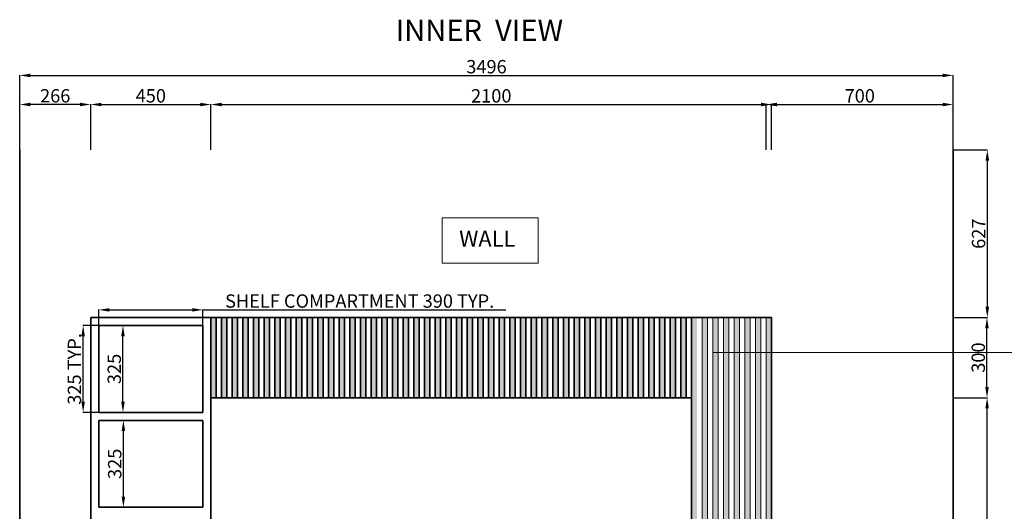
# Model space of a CAD drawing. Units: millimetres. Extents: x 11439 to 24661, y -4767 to -6.
# Tile 4 of 5: x 18965 to 22652, y -2690 to -851. Entities that reach past the tile are written whole.
import ezdxf

# ---------------------------------------------------------------- set-up
doc = ezdxf.new("R2010")
doc.units = ezdxf.units.MM
for name, color, linetype, lineweight in [('A-ANNO-DIMS', 2, 'Continuous', 18), ('A-ANNO-TEXT', 3, 'Continuous', 18), ('A-FURN', 7, 'Continuous', 35), ('A-FURN-PATT', 8, 'Continuous', 13)]:
    doc.layers.add(name, color=color, linetype=linetype, lineweight=lineweight)
doc.styles.get("Standard").update_dxf_attribs({"font": 'arial.ttf'})
doc.dimstyles.new('ISO-25', dxfattribs={"dimtxt": 50, "dimasz": 40, "dimexe": 1.25, "dimexo": 0.625, "dimtad": 1, "dimtxsty": 'Standard', "dimcen": 2.5, "dimadec": 0, "dimazin": 0, "dimtfac": 1, "dimtmove": 0, "dimatfit": 3, "dimfxl": 1, "dimarcsym": 0})

# ---------------------------------------------------------------- blocks, each defined once
blk = doc.blocks.new('*D28')
at = {"layer": 'A-ANNO-DIMS', "color": 0, "lineweight": -2, "transparency": 16777216}
for p, q in [((22461.4, -2264.7), (22588.9, -2264.7)), ((22587.6, -3424.7), (22587.6, -2304.7)), ((22461.4, -3464.7), (22588.9, -3464.7))]:
    blk.add_line(p, q, dxfattribs=at)
at = {"layer": 'A-ANNO-DIMS', "color": 0, "transparency": 16777216}
for points in [[(22581, -2304.7), (22594.3, -2304.7), (22587.6, -2264.7)], [(22581, -3424.7), (22594.3, -3424.7), (22587.6, -3464.7)]]:
    blk.add_solid(points, dxfattribs=at)
at = {"layer": 'Defpoints', "color": 0, "transparency": 16777216}
for p in [(22460.8, -2264.7), (22587.6, -2264.7), (22460.8, -3464.7)]:
    blk.add_point(p, dxfattribs=at)
at = {"layer": 'A-ANNO-DIMS', "color": 0, "transparency": 16777216, "insert": (22561.5, -2864.7), "char_height": 50, "attachment_point": 5, "rotation": 90}
blk.add_mtext('1200', dxfattribs=at)
blk = doc.blocks.new('*D29')
at = {"layer": 'A-ANNO-DIMS', "color": 0, "lineweight": -2, "transparency": 16777216}
for p, q in [((22465.2, -1964.7), (22588.5, -1964.7)), ((22587.2, -2224.7), (22587.2, -2004.7)), ((22461.4, -2264.7), (22588.5, -2264.7))]:
    blk.add_line(p, q, dxfattribs=at)
at = {"layer": 'A-ANNO-DIMS', "color": 0, "transparency": 16777216}
for points in [[(22580.5, -2004.7), (22593.9, -2004.7), (22587.2, -1964.7)], [(22580.5, -2224.7), (22593.9, -2224.7), (22587.2, -2264.7)]]:
    blk.add_solid(points, dxfattribs=at)
at = {"layer": 'Defpoints', "color": 0, "transparency": 16777216}
for p in [(22464.5, -1964.7), (22587.2, -1964.7), (22460.8, -2264.7)]:
    blk.add_point(p, dxfattribs=at)
at = {"layer": 'A-ANNO-DIMS', "color": 0, "transparency": 16777216, "insert": (22561, -2114.7), "char_height": 50, "attachment_point": 5, "rotation": 90}
blk.add_mtext('300', dxfattribs=at)
blk = doc.blocks.new('*D23')
at = {"layer": 'A-ANNO-DIMS', "color": 0, "lineweight": -2, "transparency": 16777216}
for p, q in [((18964.8, -1337.1), (18964.8, -1166.8)), ((19190.8, -1168), (19004.8, -1168)), ((19230.8, -1337.1), (19230.8, -1166.8))]:
    blk.add_line(p, q, dxfattribs=at)
at = {"layer": 'A-ANNO-DIMS', "color": 0, "transparency": 16777216}
for points in [[(19004.8, -1161.4), (19004.8, -1174.7), (18964.8, -1168)], [(19190.8, -1161.4), (19190.8, -1174.7), (19230.8, -1168)]]:
    blk.add_solid(points, dxfattribs=at)
at = {"layer": 'Defpoints', "color": 0, "transparency": 16777216}
for p in [(18964.8, -1168), (18964.8, -1337.7), (19230.8, -1337.7)]:
    blk.add_point(p, dxfattribs=at)
at = {"layer": 'A-ANNO-DIMS', "color": 0, "transparency": 16777216, "insert": (19097.8, -1141.9), "char_height": 50, "attachment_point": 5}
blk.add_mtext('266', dxfattribs=at)
blk = doc.blocks.new('*D24')
at = {"layer": 'A-ANNO-DIMS', "color": 0, "lineweight": -2, "transparency": 16777216}
for p, q in [((19230.8, -1337.1), (19230.8, -1166.8)), ((19270.8, -1168), (19640.8, -1168)), ((19680.8, -1337.1), (19680.8, -1166.8))]:
    blk.add_line(p, q, dxfattribs=at)
at = {"layer": 'A-ANNO-DIMS', "color": 0, "transparency": 16777216}
for points in [[(19270.8, -1161.4), (19270.8, -1174.7), (19230.8, -1168)], [(19640.8, -1161.4), (19640.8, -1174.7), (19680.8, -1168)]]:
    blk.add_solid(points, dxfattribs=at)
at = {"layer": 'Defpoints', "color": 0, "transparency": 16777216}
for p in [(19680.8, -1168), (19230.8, -1337.7), (19680.8, -1337.7)]:
    blk.add_point(p, dxfattribs=at)
at = {"layer": 'A-ANNO-DIMS', "color": 0, "transparency": 16777216, "insert": (19455.8, -1141.9), "char_height": 50, "attachment_point": 5}
blk.add_mtext('450', dxfattribs=at)
blk = doc.blocks.new('*D25')
at = {"layer": 'A-ANNO-DIMS', "color": 0, "lineweight": -2, "transparency": 16777216}
for p, q in [((19680.8, -1337.1), (19680.8, -1166.9)), ((19720.8, -1168.1), (21740.8, -1168.1)), ((21780.8, -1337.1), (21780.8, -1166.9))]:
    blk.add_line(p, q, dxfattribs=at)
at = {"layer": 'A-ANNO-DIMS', "color": 0, "transparency": 16777216}
for points in [[(19720.8, -1161.4), (19720.8, -1174.8), (19680.8, -1168.1)], [(21740.8, -1161.4), (21740.8, -1174.8), (21780.8, -1168.1)]]:
    blk.add_solid(points, dxfattribs=at)
at = {"layer": 'Defpoints', "color": 0, "transparency": 16777216}
for p in [(21780.8, -1168.1), (19680.8, -1337.7), (21780.8, -1337.7)]:
    blk.add_point(p, dxfattribs=at)
at = {"layer": 'A-ANNO-DIMS', "color": 0, "transparency": 16777216, "insert": (20730.8, -1142), "char_height": 50, "attachment_point": 5}
blk.add_mtext('2100', dxfattribs=at)
blk = doc.blocks.new('*D36')
at = {"layer": 'A-ANNO-DIMS', "color": 0, "lineweight": -2, "transparency": 16777216}
for p, q in [((21760.8, -1337.1), (21760.8, -1166.9)), ((21800.8, -1168.1), (22420.8, -1168.1)), ((22460.8, -1337.1), (22460.8, -1166.9))]:
    blk.add_line(p, q, dxfattribs=at)
at = {"layer": 'A-ANNO-DIMS', "color": 0, "transparency": 16777216}
for points in [[(21800.8, -1161.4), (21800.8, -1174.8), (21760.8, -1168.1)], [(22420.8, -1161.4), (22420.8, -1174.8), (22460.8, -1168.1)]]:
    blk.add_solid(points, dxfattribs=at)
at = {"layer": 'Defpoints', "color": 0, "transparency": 16777216}
for p in [(22460.8, -1168.1), (21760.8, -1337.7), (22460.8, -1337.7)]:
    blk.add_point(p, dxfattribs=at)
at = {"layer": 'A-ANNO-DIMS', "color": 0, "transparency": 16777216, "insert": (22110.8, -1142), "char_height": 50, "attachment_point": 5}
blk.add_mtext('700', dxfattribs=at)
blk = doc.blocks.new('*D30')
at = {"layer": 'A-ANNO-DIMS', "color": 0, "lineweight": -2, "transparency": 16777216}
for p, q in [((22461.4, -1337.7), (22589.7, -1337.7)), ((22588.5, -1377.7), (22588.5, -1924.7)), ((22465.2, -1964.7), (22589.7, -1964.7))]:
    blk.add_line(p, q, dxfattribs=at)
at = {"layer": 'A-ANNO-DIMS', "color": 0, "transparency": 16777216}
for points in [[(22581.8, -1377.7), (22595.1, -1377.7), (22588.5, -1337.7)], [(22581.8, -1924.7), (22595.1, -1924.7), (22588.5, -1964.7)]]:
    blk.add_solid(points, dxfattribs=at)
at = {"layer": 'Defpoints', "color": 0, "transparency": 16777216}
for p in [(22460.8, -1337.7), (22464.5, -1964.7), (22588.5, -1964.7)]:
    blk.add_point(p, dxfattribs=at)
at = {"layer": 'A-ANNO-DIMS', "color": 0, "transparency": 16777216, "insert": (22562.3, -1651.2), "char_height": 50, "attachment_point": 5, "rotation": 90}
blk.add_mtext('627', dxfattribs=at)
blk = doc.blocks.new('*D41')
at = {"layer": 'A-ANNO-DIMS', "color": 0, "lineweight": -2, "transparency": 16777216}
for p, q in [((19261.4, -2349.7), (19354.4, -2349.7)), ((19353.1, -2634.7), (19353.1, -2389.7)), ((19261.4, -2674.7), (19354.4, -2674.7))]:
    blk.add_line(p, q, dxfattribs=at)
at = {"layer": 'A-ANNO-DIMS', "color": 0, "transparency": 16777216}
for points in [[(19346.5, -2389.7), (19359.8, -2389.7), (19353.1, -2349.7)], [(19346.5, -2634.7), (19359.8, -2634.7), (19353.1, -2674.7)]]:
    blk.add_solid(points, dxfattribs=at)
at = {"layer": 'Defpoints', "color": 0, "transparency": 16777216}
for p in [(19260.8, -2349.7), (19353.1, -2349.7), (19260.8, -2674.7)]:
    blk.add_point(p, dxfattribs=at)
at = {"layer": 'A-ANNO-DIMS', "color": 0, "transparency": 16777216, "insert": (19327, -2512.2), "char_height": 50, "attachment_point": 5, "rotation": 90}
blk.add_mtext('325', dxfattribs=at)
blk = doc.blocks.new('*D42')
at = {"layer": 'A-ANNO-DIMS', "color": 0, "lineweight": -2, "transparency": 16777216}
for p, q in [((19261.4, -1994.7), (19352.7, -1994.7)), ((19351.5, -2279.7), (19351.5, -2034.7)), ((19261.4, -2319.7), (19352.7, -2319.7))]:
    blk.add_line(p, q, dxfattribs=at)
at = {"layer": 'A-ANNO-DIMS', "color": 0, "transparency": 16777216}
for points in [[(19344.8, -2034.7), (19358.2, -2034.7), (19351.5, -1994.7)], [(19344.8, -2279.7), (19358.2, -2279.7), (19351.5, -2319.7)]]:
    blk.add_solid(points, dxfattribs=at)
at = {"layer": 'Defpoints', "color": 0, "transparency": 16777216}
for p in [(19260.8, -1994.7), (19351.5, -1994.7), (19260.8, -2319.7)]:
    blk.add_point(p, dxfattribs=at)
at = {"layer": 'A-ANNO-DIMS', "color": 0, "transparency": 16777216, "insert": (19325.3, -2157.2), "char_height": 50, "attachment_point": 5, "rotation": 90}
blk.add_mtext('325', dxfattribs=at)
blk = doc.blocks.new('SHELF-COMPARTMENT')
for p, q in [((0, 325), (390, 325)), ((0, 0), (0, 325)), ((390, 0), (390, 325)), ((0, 0), (390, 0))]:
    blk.add_line(p, q)
blk = doc.blocks.new('*D47')
at = {"layer": 'A-ANNO-DIMS', "color": 0, "lineweight": -2, "transparency": 16777216}
for p, q in [((19260.8, -1994.1), (19260.8, -1934.9)), ((19300.8, -1936.2), (19610.8, -1936.2)), ((19650.8, -1994.1), (19650.8, -1934.9)), ((19650.8, -1936.2), (20785.1, -1936.2))]:
    blk.add_line(p, q, dxfattribs=at)
at = {"layer": 'A-ANNO-DIMS', "color": 0, "transparency": 16777216}
for points in [[(19300.8, -1929.5), (19300.8, -1942.9), (19260.8, -1936.2)], [(19610.8, -1929.5), (19610.8, -1942.9), (19650.8, -1936.2)]]:
    blk.add_solid(points, dxfattribs=at)
at = {"layer": 'Defpoints', "color": 0, "transparency": 16777216}
for p in [(19650.8, -1936.2), (19260.8, -1994.7), (19650.8, -1994.7)]:
    blk.add_point(p, dxfattribs=at)
at = {"layer": 'A-ANNO-DIMS', "color": 0, "transparency": 16777216, "insert": (20237.9, -1909.7), "char_height": 50, "attachment_point": 5}
blk.add_mtext('SHELF COMPARTMENT 390 TYP.', dxfattribs=at)
blk = doc.blocks.new('*D48')
at = {"layer": 'A-ANNO-DIMS', "color": 0, "lineweight": -2, "transparency": 16777216}
for p, q in [((19260.1, -1994.7), (19201, -1994.7)), ((19202.3, -2279.7), (19202.3, -2034.7)), ((19260.1, -2319.7), (19201, -2319.7))]:
    blk.add_line(p, q, dxfattribs=at)
at = {"layer": 'A-ANNO-DIMS', "color": 0, "transparency": 16777216}
for points in [[(19195.6, -2034.7), (19208.9, -2034.7), (19202.3, -1994.7)], [(19195.6, -2279.7), (19208.9, -2279.7), (19202.3, -2319.7)]]:
    blk.add_solid(points, dxfattribs=at)
at = {"layer": 'Defpoints', "color": 0, "transparency": 16777216}
for p in [(19202.3, -1994.7), (19260.8, -1994.7), (19260.8, -2319.7)]:
    blk.add_point(p, dxfattribs=at)
at = {"layer": 'A-ANNO-DIMS', "color": 0, "transparency": 16777216, "insert": (19176.1, -2157.2), "char_height": 50, "attachment_point": 5, "rotation": 90}
blk.add_mtext('325 TYP.', dxfattribs=at)
blk = doc.blocks.new('*D60')
at = {"layer": 'A-ANNO-DIMS', "color": 0, "lineweight": -2, "transparency": 16777216}
for p, q in [((18964.8, -1337.1), (18964.8, -1057.9)), ((19004.8, -1059.2), (22420.8, -1059.2)), ((22460.8, -1337.1), (22460.8, -1057.9))]:
    blk.add_line(p, q, dxfattribs=at)
at = {"layer": 'A-ANNO-DIMS', "color": 0, "transparency": 16777216}
for points in [[(19004.8, -1052.5), (19004.8, -1065.9), (18964.8, -1059.2)], [(22420.8, -1052.5), (22420.8, -1065.9), (22460.8, -1059.2)]]:
    blk.add_solid(points, dxfattribs=at)
at = {"layer": 'Defpoints', "color": 0, "transparency": 16777216}
for p in [(22460.8, -1059.2), (18964.8, -1337.7), (22460.8, -1337.7)]:
    blk.add_point(p, dxfattribs=at)
at = {"layer": 'A-ANNO-DIMS', "color": 0, "transparency": 16777216, "insert": (20712.8, -1033), "char_height": 50, "attachment_point": 5}
blk.add_mtext('3496', dxfattribs=at)

msp = doc.modelspace()

# ---------------------------------------------------------------- hatches: boundary and pattern name
at = {"layer": 'A-FURN-PATT'}
h = msp.add_hatch(color=256, dxfattribs=at)
h.dxf.hatch_style = 1
h.paths.add_polyline_path([(19700.761, -3464.684), (19680.761, -3464.684), (19680.761, -3764.684), (19700.761, -3764.684)])
h.paths.add_polyline_path([(19740.761, -3464.684), (19720.761, -3464.684), (19720.761, -3764.684), (19740.761, -3764.684)])
h.paths.add_polyline_path([(19780.761, -3464.684), (19760.761, -3464.684), (19760.761, -3764.684), (19780.761, -3764.684)])
h.paths.add_polyline_path([(19800.761, -3764.684), (19820.761, -3764.684), (19820.761, -3464.684), (19800.761, -3464.684)])
h.paths.add_polyline_path([(19860.761, -3464.684), (19840.761, -3464.684), (19840.761, -3764.684), (19860.761, -3764.684)])
h.paths.add_polyline_path([(19900.761, -3464.684), (19880.761, -3464.684), (19880.761, -3764.684), (19900.761, -3764.684)])
h.paths.add_polyline_path([(19940.761, -3464.684), (19920.761, -3464.684), (19920.761, -3764.684), (19940.761, -3764.684)])
h.paths.add_polyline_path([(19960.761, -3764.684), (19980.761, -3764.684), (19980.761, -3464.684), (19960.761, -3464.684)])
h.paths.add_polyline_path([(20020.761, -3464.684), (20000.761, -3464.684), (20000.761, -3764.684), (20020.761, -3764.684)])
h.paths.add_polyline_path([(20040.761, -3764.684), (20060.761, -3764.684), (20060.761, -3464.684), (20040.761, -3464.684)])
h.paths.add_polyline_path([(20080.761, -3764.684), (20100.761, -3764.684), (20100.761, -3464.684), (20080.761, -3464.684)])
h.paths.add_polyline_path([(20140.761, -3464.684), (20120.761, -3464.684), (20120.761, -3764.684), (20140.761, -3764.684)])
h.paths.add_polyline_path([(20160.761, -3764.684), (20180.761, -3764.684), (20180.761, -3464.684), (20160.761, -3464.684)])
h.paths.add_polyline_path([(20220.761, -3464.684), (20200.761, -3464.684), (20200.761, -3764.684), (20220.761, -3764.684)])
h.paths.add_polyline_path([(20240.761, -3764.684), (20260.761, -3764.684), (20260.761, -3464.684), (20240.761, -3464.684)])
h.paths.add_polyline_path([(20300.761, -3464.684), (20280.761, -3464.684), (20280.761, -3764.684), (20300.761, -3764.684)])
h.paths.add_polyline_path([(20340.761, -3464.684), (20320.761, -3464.684), (20320.761, -3764.684), (20340.761, -3764.684)])
h.paths.add_polyline_path([(20360.761, -3764.684), (20380.761, -3764.684), (20380.761, -3464.684), (20360.761, -3464.684)])
h.paths.add_polyline_path([(20400.761, -3764.684), (20420.761, -3764.684), (20420.761, -3464.684), (20400.761, -3464.684)])
h.paths.add_polyline_path([(20440.761, -3764.684), (20460.761, -3764.684), (20460.761, -3464.684), (20440.761, -3464.684)])
h.paths.add_polyline_path([(20480.761, -3764.684), (20500.761, -3764.684), (20500.761, -3464.684), (20480.761, -3464.684)])
h.paths.add_polyline_path([(20520.761, -3764.684), (20540.761, -3764.684), (20540.761, -3464.684), (20520.761, -3464.684)])
h.paths.add_polyline_path([(20560.761, -3764.684), (20580.761, -3764.684), (20580.761, -3464.684), (20560.761, -3464.684)])
h.paths.add_polyline_path([(20600.761, -3764.684), (20620.761, -3764.684), (20620.761, -3464.684), (20600.761, -3464.684)])
h.paths.add_polyline_path([(20660.761, -3464.684), (20640.761, -3464.684), (20640.761, -3764.684), (20660.761, -3764.684)])
h.paths.add_polyline_path([(20680.761, -3764.684), (20700.761, -3764.684), (20700.761, -3464.684), (20680.761, -3464.684)])
h.paths.add_polyline_path([(20740.761, -3464.684), (20720.761, -3464.684), (20720.761, -3764.684), (20740.761, -3764.684)])
h.paths.add_polyline_path([(20760.761, -3764.684), (20780.761, -3764.684), (20780.761, -3464.684), (20760.761, -3464.684)])
h.paths.add_polyline_path([(20800.761, -3764.684), (20820.761, -3764.684), (20820.761, -3464.684), (20800.761, -3464.684)])
h.paths.add_polyline_path([(20840.761, -3764.684), (20860.761, -3764.684), (20860.761, -3464.684), (20840.761, -3464.684)])
h.paths.add_polyline_path([(20900.761, -3464.684), (20880.761, -3464.684), (20880.761, -3764.684), (20900.761, -3764.684)])
h.paths.add_polyline_path([(20940.761, -3464.684), (20920.761, -3464.684), (20920.761, -3764.684), (20940.761, -3764.684)])
h.paths.add_polyline_path([(20980.761, -3464.684), (20960.761, -3464.684), (20960.761, -3764.684), (20980.761, -3764.684)])
h.paths.add_polyline_path([(21020.761, -3464.684), (21000.761, -3464.684), (21000.761, -3764.684), (21020.761, -3764.684)])
h.paths.add_polyline_path([(21060.761, -3464.684), (21040.761, -3464.684), (21040.761, -3764.684), (21060.761, -3764.684)])
h.paths.add_polyline_path([(21080.761, -3764.684), (21100.761, -3764.684), (21100.761, -3464.684), (21080.761, -3464.684)])
h.paths.add_polyline_path([(21120.761, -3764.684), (21140.761, -3764.684), (21140.761, -3464.684), (21120.761, -3464.684)])
h.paths.add_polyline_path([(21180.761, -3464.684), (21160.761, -3464.684), (21160.761, -3764.684), (21180.761, -3764.684)])
h.paths.add_polyline_path([(21200.761, -3764.684), (21220.761, -3764.684), (21220.761, -3464.684), (21200.761, -3464.684)])
h.paths.add_polyline_path([(21260.761, -3464.684), (21240.761, -3464.684), (21240.761, -3764.684), (21260.761, -3764.684)])
h.paths.add_polyline_path([(21280.761, -3764.684), (21300.761, -3764.684), (21300.761, -3464.684), (21280.761, -3464.684)])
h.paths.add_polyline_path([(21320.761, -3764.684), (21340.761, -3764.684), (21340.761, -3464.684), (21320.761, -3464.684)])
h.paths.add_polyline_path([(21360.761, -3764.684), (21380.761, -3764.684), (21380.761, -3464.684), (21360.761, -3464.684)])
h.paths.add_polyline_path([(21400.761, -3764.684), (21420.761, -3764.684), (21420.761, -3464.684), (21400.761, -3464.684)])
h.paths.add_polyline_path([(21460.761, -3464.684), (21440.761, -3464.684), (21440.761, -3764.684), (21460.761, -3764.684)])
h.paths.add_polyline_path([(19700.761, -1964.684), (19680.761, -1964.684), (19680.761, -2264.684), (19700.761, -2264.684)])
h.paths.add_polyline_path([(19740.761, -1964.684), (19720.761, -1964.684), (19720.761, -2264.684), (19740.761, -2264.684)])
h.paths.add_polyline_path([(19780.761, -1964.684), (19760.761, -1964.684), (19760.761, -2264.684), (19780.761, -2264.684)])
h.paths.add_polyline_path([(19820.761, -1964.684), (19800.761, -1964.684), (19800.761, -2264.684), (19820.761, -2264.684)])
h.paths.add_polyline_path([(19860.761, -2264.684), (19860.761, -1964.684), (19840.761, -1964.684), (19840.761, -2264.684)])
h.paths.add_polyline_path([(19880.761, -2264.684), (19900.761, -2264.684), (19900.761, -1964.684), (19880.761, -1964.684)])
h.paths.add_polyline_path([(19940.761, -1964.684), (19920.761, -1964.684), (19920.761, -2264.684), (19940.761, -2264.684)])
h.paths.add_polyline_path([(19960.761, -2264.684), (19980.761, -2264.684), (19980.761, -1964.684), (19960.761, -1964.684)])
h.paths.add_polyline_path([(20020.761, -1964.684), (20000.761, -1964.684), (20000.761, -2264.684), (20020.761, -2264.684)])
h.paths.add_polyline_path([(20040.761, -2264.684), (20060.761, -2264.684), (20060.761, -1964.684), (20040.761, -1964.684)])
h.paths.add_polyline_path([(20100.761, -1964.684), (20080.761, -1964.684), (20080.761, -2264.684), (20100.761, -2264.684)])
h.paths.add_polyline_path([(20120.761, -2264.684), (20140.761, -2264.684), (20140.761, -1964.684), (20120.761, -1964.684)])
h.paths.add_polyline_path([(20180.761, -1964.684), (20160.761, -1964.684), (20160.761, -2264.684), (20180.761, -2264.684)])
h.paths.add_polyline_path([(20220.761, -1964.684), (20200.761, -1964.684), (20200.761, -2264.684), (20220.761, -2264.684)])
h.paths.add_polyline_path([(20240.761, -2264.684), (20260.761, -2264.684), (20260.761, -1964.684), (20240.761, -1964.684)])
h.paths.add_polyline_path([(20280.761, -2264.684), (20300.761, -2264.684), (20300.761, -1964.684), (20280.761, -1964.684)])
h.paths.add_polyline_path([(20340.761, -1964.684), (20320.761, -1964.684), (20320.761, -2264.684), (20340.761, -2264.684)])
h.paths.add_polyline_path([(20360.761, -2264.684), (20380.761, -2264.684), (20380.761, -1964.684), (20360.761, -1964.684)])
h.paths.add_polyline_path([(20400.761, -2264.684), (20420.761, -2264.684), (20420.761, -1964.684), (20400.761, -1964.684)])
h.paths.add_polyline_path([(20440.761, -2264.684), (20460.761, -2264.684), (20460.761, -1964.684), (20440.761, -1964.684)])
h.paths.add_polyline_path([(20480.761, -2264.684), (20500.761, -2264.684), (20500.761, -1964.684), (20480.761, -1964.684)])
h.paths.add_polyline_path([(20520.761, -2264.684), (20540.761, -2264.684), (20540.761, -1964.684), (20520.761, -1964.684)])
h.paths.add_polyline_path([(20580.761, -1964.684), (20560.761, -1964.684), (20560.761, -2264.684), (20580.761, -2264.684)])
h.paths.add_polyline_path([(20600.761, -2264.684), (20620.761, -2264.684), (20620.761, -1964.684), (20600.761, -1964.684)])
h.paths.add_polyline_path([(20640.761, -2264.684), (20660.761, -2264.684), (20660.761, -1964.684), (20640.761, -1964.684)])
h.paths.add_polyline_path([(20680.761, -2264.684), (20700.761, -2264.684), (20700.761, -1964.684), (20680.761, -1964.684)])
h.paths.add_polyline_path([(20720.761, -2264.684), (20740.761, -2264.684), (20740.761, -1964.684), (20720.761, -1964.684)])
h.paths.add_polyline_path([(20780.761, -1964.684), (20760.761, -1964.684), (20760.761, -2264.684), (20780.761, -2264.684)])
h.paths.add_polyline_path([(20800.761, -2264.684), (20820.761, -2264.684), (20820.761, -1964.684), (20800.761, -1964.684)])
h.paths.add_polyline_path([(20860.761, -1964.684), (20840.761, -1964.684), (20840.761, -2264.684), (20860.761, -2264.684)])
h.paths.add_polyline_path([(20900.761, -1964.684), (20880.761, -1964.684), (20880.761, -2264.684), (20900.761, -2264.684)])
h.paths.add_polyline_path([(20940.761, -1964.684), (20920.761, -1964.684), (20920.761, -2264.684), (20940.761, -2264.684)])
h.paths.add_polyline_path([(20980.761, -1964.684), (20960.761, -1964.684), (20960.761, -2264.684), (20980.761, -2264.684)])
h.paths.add_polyline_path([(21020.761, -1964.684), (21000.761, -1964.684), (21000.761, -2264.684), (21020.761, -2264.684)])
h.paths.add_polyline_path([(21040.761, -2264.684), (21060.761, -2264.684), (21060.761, -1964.684), (21040.761, -1964.684)])
h.paths.add_polyline_path([(21080.761, -2264.684), (21100.761, -2264.684), (21100.761, -1964.684), (21080.761, -1964.684)])
h.paths.add_polyline_path([(21120.761, -2264.684), (21140.761, -2264.684), (21140.761, -1964.684), (21120.761, -1964.684)])
h.paths.add_polyline_path([(21180.761, -1964.684), (21160.761, -1964.684), (21160.761, -2264.684), (21180.761, -2264.684)])
h.paths.add_polyline_path([(21200.761, -2264.684), (21220.761, -2264.684), (21220.761, -1964.684), (21200.761, -1964.684)])
h.paths.add_polyline_path([(21240.761, -2264.684), (21260.761, -2264.684), (21260.761, -1964.684), (21240.761, -1964.684)])
h.paths.add_polyline_path([(21300.761, -1964.684), (21280.761, -1964.684), (21280.761, -2264.684), (21300.761, -2264.684)])
h.paths.add_polyline_path([(21320.761, -2264.684), (21340.761, -2264.684), (21340.761, -1964.684), (21320.761, -1964.684)])
h.paths.add_polyline_path([(21360.761, -2264.684), (21380.761, -2264.684), (21380.761, -1964.684), (21360.761, -1964.684)])
h.paths.add_polyline_path([(21400.761, -2264.684), (21420.761, -2264.684), (21420.761, -1964.684), (21400.761, -1964.684)])
h.paths.add_polyline_path([(21440.761, -2264.684), (21460.761, -2264.684), (21460.761, -1964.684), (21440.761, -1964.684)])
h = msp.add_hatch(color=256, dxfattribs=at)
h.dxf.hatch_style = 1
h.paths.add_polyline_path([(21500.761, -2881.594), (21480.761, -2881.594), (21480.761, -3464.684), (21480.761, -3764.684), (21500.761, -3764.684)])
h.paths.add_polyline_path([(21540.761, -2881.594), (21520.761, -2881.594), (21520.761, -3764.684), (21540.761, -3764.684)])
h.paths.add_polyline_path([(21580.761, -2881.594), (21560.761, -2881.594), (21560.761, -3764.684), (21580.761, -3764.684)])
h.paths.add_polyline_path([(21620.761, -2881.594), (21600.761, -2881.594), (21600.761, -3764.684), (21620.761, -3764.684)])
h.paths.add_polyline_path([(21660.761, -2881.594), (21640.761, -2881.594), (21640.761, -3764.684), (21660.761, -3764.684)])
h.paths.add_polyline_path([(21700.761, -2881.594), (21680.761, -2881.594), (21680.761, -3764.684), (21700.761, -3764.684)])
h.paths.add_polyline_path([(21740.761, -2881.594), (21720.761, -2881.594), (21720.761, -3764.684), (21740.761, -3764.684)])
h.paths.add_polyline_path([(21780.761, -2881.594), (21760.761, -2881.594), (21760.761, -3764.684), (21780.761, -3764.684)])
h.paths.add_polyline_path([(21500.761, -1964.684), (21480.761, -1964.684), (21480.761, -2264.684), (21480.761, -2881.594), (21500.761, -2881.594)])
h.paths.add_polyline_path([(21540.761, -1964.684), (21520.761, -1964.684), (21520.761, -2881.594), (21540.761, -2881.594)])
h.paths.add_polyline_path([(21580.761, -2095.642), (21560.761, -2095.642), (21560.761, -2881.594), (21580.761, -2881.594)])
h.paths.add_polyline_path([(21620.761, -2095.642), (21600.761, -2095.642), (21600.761, -2881.594), (21620.761, -2881.594)])
h.paths.add_polyline_path([(21660.761, -2095.642), (21640.761, -2095.642), (21640.761, -2881.594), (21660.761, -2881.594)])
h.paths.add_polyline_path([(21700.761, -2095.642), (21680.761, -2095.642), (21680.761, -2881.594), (21700.761, -2881.594)])
h.paths.add_polyline_path([(21740.761, -2095.642), (21720.761, -2095.642), (21720.761, -2881.594), (21740.761, -2881.594)])
h.paths.add_polyline_path([(21780.761, -2095.642), (21760.761, -2095.642), (21760.761, -2881.594), (21780.761, -2881.594)])
h = msp.add_hatch(dxfattribs=at)
h.set_pattern_fill('ANSI31', color=256, scale=6.29921, angle=45, style=0)
h.paths.add_polyline_path([(21500.761, -3798.504), (21760.761, -3798.504), (21760.761, -1964.684), (21500.761, -1964.684)])
h = msp.add_hatch(color=256, dxfattribs=at)
h.dxf.hatch_style = 1
h.paths.add_polyline_path([(21580.761, -1964.684), (21560.761, -1964.684), (21560.761, -2095.642), (21580.761, -2095.642)])
h.paths.add_polyline_path([(21620.761, -1964.684), (21600.761, -1964.684), (21600.761, -2095.642), (21620.761, -2095.642)])
h.paths.add_polyline_path([(21660.761, -1964.684), (21640.761, -1964.684), (21640.761, -2095.642), (21660.761, -2095.642)])
h.paths.add_polyline_path([(21700.761, -1964.684), (21680.761, -1964.684), (21680.761, -2095.642), (21700.761, -2095.642)])
h.paths.add_polyline_path([(21740.761, -1964.684), (21720.761, -1964.684), (21720.761, -2095.642), (21740.761, -2095.642)])
h.paths.add_polyline_path([(21780.761, -1964.684), (21760.761, -1964.684), (21760.761, -2095.642), (21780.761, -2095.642)])

# ---------------------------------------------------------------- linework, layer by layer
at = {"layer": 'A-ANNO-TEXT'}
for q in [(21560.761, -2095.642), (22907.534, -2095.642)]:
    msp.add_line((21560.761, -2095.642), q, dxfattribs=at)
msp.add_lwpolyline([(20547.212, -1592.04), (20906.598, -1592.04), (20906.598, -1761.361), (20547.212, -1761.361)], close=True, dxfattribs=at)
at = {"layer": 'A-FURN'}
for p, q in [((18964.761, -1337.684), (18964.761, -4147.684)), ((22460.761, -4147.684), (22460.761, -1337.684)), ((19230.761, -1964.684), (21780.761, -1964.684)), ((19230.761, -4147.684), (19230.761, -1964.684)), ((19680.761, -4147.684), (19680.761, -1964.684)), ((19680.761, -2264.684), (19680.761, -1964.684)), ((19700.761, -2264.684), (19700.761, -1964.684)), ((19720.761, -2264.684), (19720.761, -1964.684)), ((19740.761, -2264.684), (19740.761, -1964.684)), ((19760.761, -2264.684), (19760.761, -1964.684)), ((19780.761, -2264.684), (19780.761, -1964.684)), ((19800.761, -2264.684), (19800.761, -1964.684)), ((19820.761, -2264.684), (19820.761, -1964.684)), ((19840.761, -2264.684), (19840.761, -1964.684)), ((19860.761, -2264.684), (19860.761, -1964.684)), ((19880.761, -2264.684), (19880.761, -1964.684)), ((19900.761, -2264.684), (19900.761, -1964.684)), ((19920.761, -2264.684), (19920.761, -1964.684)), ((19940.761, -2264.684), (19940.761, -1964.684)), ((19960.761, -2264.684), (19960.761, -1964.684)), ((19980.761, -2264.684), (19980.761, -1964.684)), ((20000.761, -2264.684), (20000.761, -1964.684)), ((20020.761, -2264.684), (20020.761, -1964.684)), ((20040.761, -2264.684), (20040.761, -1964.684)), ((20060.761, -2264.684), (20060.761, -1964.684)), ((20080.761, -2264.684), (20080.761, -1964.684)), ((20100.761, -2264.684), (20100.761, -1964.684)), ((20120.761, -2264.684), (20120.761, -1964.684)), ((20140.761, -2264.684), (20140.761, -1964.684)), ((20160.761, -2264.684), (20160.761, -1964.684)), ((20180.761, -2264.684), (20180.761, -1964.684)), ((20200.761, -2264.684), (20200.761, -1964.684)), ((20220.761, -2264.684), (20220.761, -1964.684)), ((20240.761, -2264.684), (20240.761, -1964.684)), ((20260.761, -2264.684), (20260.761, -1964.684)), ((20280.761, -2264.684), (20280.761, -1964.684)), ((20300.761, -2264.684), (20300.761, -1964.684)), ((20320.761, -2264.684), (20320.761, -1964.684)), ((20340.761, -2264.684), (20340.761, -1964.684)), ((20360.761, -2264.684), (20360.761, -1964.684)), ((20380.761, -2264.684), (20380.761, -1964.684)), ((20400.761, -2264.684), (20400.761, -1964.684)), ((20420.761, -2264.684), (20420.761, -1964.684)), ((20440.761, -2264.684), (20440.761, -1964.684)), ((20460.761, -2264.684), (20460.761, -1964.684)), ((20480.761, -2264.684), (20480.761, -1964.684)), ((20500.761, -2264.684), (20500.761, -1964.684)), ((20520.761, -2264.684), (20520.761, -1964.684)), ((20540.761, -2264.684), (20540.761, -1964.684)), ((20560.761, -2264.684), (20560.761, -1964.684)), ((20580.761, -2264.684), (20580.761, -1964.684)), ((20600.761, -2264.684), (20600.761, -1964.684)), ((20620.761, -2264.684), (20620.761, -1964.684)), ((20640.761, -2264.684), (20640.761, -1964.684)), ((20660.761, -2264.684), (20660.761, -1964.684)), ((20680.761, -2264.684), (20680.761, -1964.684)), ((20700.761, -2264.684), (20700.761, -1964.684)), ((20720.761, -2264.684), (20720.761, -1964.684)), ((20740.761, -2264.684), (20740.761, -1964.684)), ((20760.761, -2264.684), (20760.761, -1964.684)), ((20780.761, -2264.684), (20780.761, -1964.684)), ((20800.761, -2264.684), (20800.761, -1964.684)), ((20820.761, -2264.684), (20820.761, -1964.684)), ((20840.761, -2264.684), (20840.761, -1964.684)), ((20860.761, -2264.684), (20860.761, -1964.684)), ((20880.761, -2264.684), (20880.761, -1964.684)), ((20900.761, -2264.684), (20900.761, -1964.684)), ((20920.761, -2264.684), (20920.761, -1964.684)), ((20940.761, -2264.684), (20940.761, -1964.684)), ((20960.761, -2264.684), (20960.761, -1964.684)), ((20980.761, -2264.684), (20980.761, -1964.684)), ((21000.761, -2264.684), (21000.761, -1964.684)), ((21020.761, -2264.684), (21020.761, -1964.684)), ((21040.761, -2264.684), (21040.761, -1964.684)), ((21060.761, -2264.684), (21060.761, -1964.684)), ((21080.761, -2264.684), (21080.761, -1964.684)), ((21100.761, -2264.684), (21100.761, -1964.684)), ((21120.761, -2264.684), (21120.761, -1964.684)), ((21140.761, -2264.684), (21140.761, -1964.684)), ((21160.761, -2264.684), (21160.761, -1964.684)), ((21180.761, -2264.684), (21180.761, -1964.684)), ((21200.761, -2264.684), (21200.761, -1964.684)), ((21220.761, -2264.684), (21220.761, -1964.684)), ((21240.761, -2264.684), (21240.761, -1964.684)), ((21260.761, -2264.684), (21260.761, -1964.684)), ((21280.761, -2264.684), (21280.761, -1964.684)), ((21300.761, -2264.684), (21300.761, -1964.684)), ((21320.761, -2264.684), (21320.761, -1964.684)), ((21340.761, -2264.684), (21340.761, -1964.684)), ((21360.761, -2264.684), (21360.761, -1964.684)), ((21380.761, -2264.684), (21380.761, -1964.684)), ((21400.761, -2264.684), (21400.761, -1964.684)), ((21420.761, -2264.684), (21420.761, -1964.684)), ((21440.761, -2264.684), (21440.761, -1964.684)), ((21460.761, -2264.684), (21460.761, -1964.684)), ((21480.761, -2264.684), (21480.761, -1964.684)), ((21780.761, -4147.684), (21780.761, -1964.684)), ((19680.761, -2264.684), (21480.761, -2264.684)), ((21480.761, -3464.684), (21480.761, -2264.684))]:
    msp.add_line(p, q, dxfattribs=at)

# ---------------------------------------------------------------- block references
msp.add_blockref('SHELF-COMPARTMENT', (19260.761, -2319.684), dxfattribs=at)
at = {"layer": 'A-FURN', "rotation": 180}
msp.add_blockref('SHELF-COMPARTMENT', (19650.761, -2349.685), dxfattribs=at)

# ---------------------------------------------------------------- texts
at = {"layer": 'A-ANNO-TEXT', "attachment_point": 1}
for s, insert, char_height in [('INNER  VIEW', (20372.716, -850.809), 80), ('WALL', (20610.532, -1639.929), 60)]:
    msp.add_mtext_dynamic_manual_height_columns(s, width=1074.7282, gutter_width=12.5, heights=[0], dxfattribs=dict(at, insert=insert, char_height=char_height))

# ---------------------------------------------------------------- dimensions: what is measured, and where the dimension line sits
at = {"layer": 'A-ANNO-DIMS'}
for base, p1, p2, override, picture, middle in [((22460.761, -1059.184), (18964.761, -1337.684), (22460.761, -1337.684), {"dimdec": 0, "dimlfac": 1, "dimrnd": 0, "dimzin": 0, "dimdsep": 46, "dimlunit": 2}, '*D60', (20712.761, -1033.014)), ((18964.761, -1168.021), (19230.761, -1337.684), (18964.761, -1337.684), {"dimclrd": 0, "dimclre": 0, "dimclrt": 0}, '*D23', (19097.761, -1141.867)), ((19680.761, -1168.021), (19230.761, -1337.684), (19680.761, -1337.684), {"dimclrd": 0, "dimclre": 0, "dimclrt": 0}, '*D24', (19455.761, -1141.867)), ((21780.761, -1168.113), (19680.761, -1337.684), (21780.761, -1337.684), {"dimclrd": 0, "dimclre": 0, "dimclrt": 0}, '*D25', (20730.761, -1141.959)), ((22460.761, -1168.113), (21760.761, -1337.684), (22460.761, -1337.684), {"dimclrd": 0, "dimclre": 0, "dimclrt": 0}, '*D36', (22110.761, -1141.959))]:
    dim = msp.add_linear_dim(base=base, p1=p1, p2=p2, dimstyle='ISO-25', override=override, dxfattribs=at)
    dim.commit()
    dim.dimension.update_dxf_attribs({"geometry": picture, "text_midpoint": middle})
for base, p1, p2, picture, middle in [((22588.452, -1964.684), (22460.761, -1337.684), (22464.536, -1964.684), '*D30', (22562.299, -1651.184)), ((22587.202, -1964.684), (22460.761, -2264.684), (22464.536, -1964.684), '*D29', (22561.032, -2114.684)), ((19351.496, -1994.684), (19260.761, -2319.684), (19260.761, -1994.684), '*D42', (19325.325, -2157.184)), ((22587.626, -2264.684), (22460.761, -3464.684), (22460.761, -2264.684), '*D28', (22561.472, -2864.684))]:
    dim = msp.add_linear_dim(base=base, p1=p1, p2=p2, angle=90, dimstyle='ISO-25', override={"dimclrd": 0, "dimclre": 0, "dimclrt": 0}, dxfattribs=at)
    dim.commit()
    dim.dimension.update_dxf_attribs({"geometry": picture, "text_midpoint": middle})
dim = msp.add_linear_dim(base=(19650.761, -1936.184), p1=(19260.761, -1994.684), p2=(19650.761, -1994.684), text='SHELF COMPARTMENT <> TYP.', dimstyle='ISO-25', override={"dimdec": 0, "dimrnd": 0, "dimzin": 0, "dimlunit": 2}, dxfattribs=at)
dim.commit()
dim.dimension.update_dxf_attribs({"geometry": '*D47', "text_midpoint": (20237.924, -1909.673)})
dim = msp.add_linear_dim(base=(19202.261, -1994.684), p1=(19260.761, -2319.684), p2=(19260.761, -1994.684), angle=90, text='<> TYP.', dimstyle='ISO-25', override={"dimdec": 0, "dimrnd": 0, "dimzin": 0, "dimlunit": 2}, dxfattribs=at)
dim.commit()
dim.dimension.update_dxf_attribs({"geometry": '*D48', "text_midpoint": (19176.09, -2157.184)})
dim = msp.add_aligned_dim(p1=(19260.761, -2674.684), p2=(19260.761, -2349.684), distance=-92.363, dimstyle='ISO-25', override={"dimclrd": 0, "dimclre": 0, "dimclrt": 0}, dxfattribs=at)
dim.commit()
dim.dimension.update_dxf_attribs({"geometry": '*D41', "text_midpoint": (19326.953, -2512.184)})

doc.saveas('drawing.dxf')
